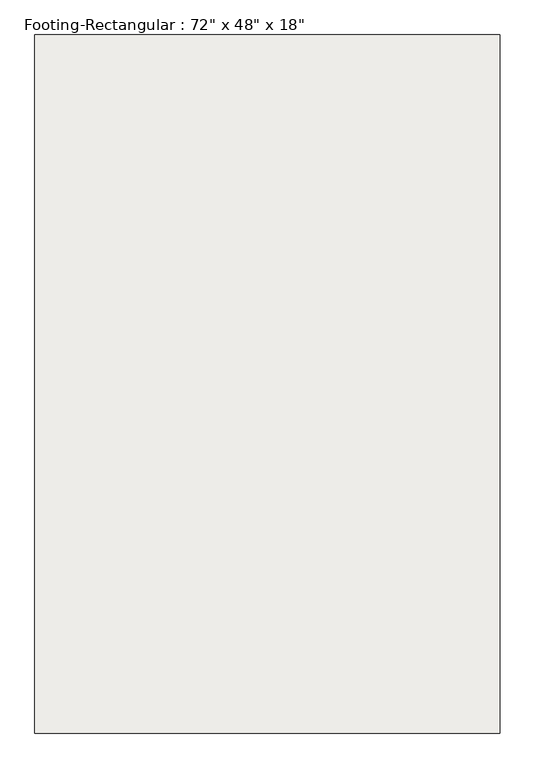
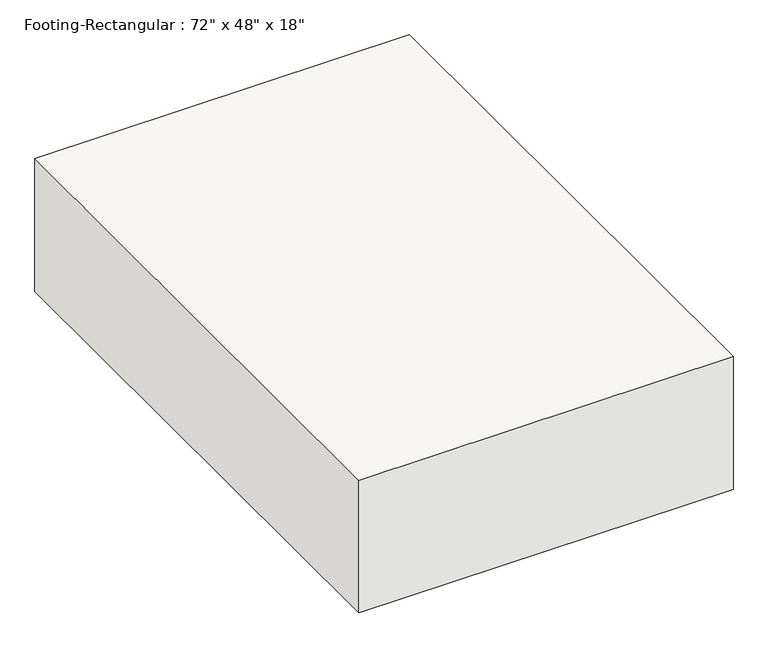
"""IFC4 building model written with IfcOpenShell, lengths in millimetres: slab geometry."""

from ifc_helpers import new_model, si_unit, frame, origin, place, context, project, spatial, polyline, outline, extrude, source, transform, mapped, element, save


def slab_5ba74754(model_context):
    return source(origin(), model_context, "Body", "SweptSolid", [
        extrude(outline(polyline([(609.6, 914.4), (609.6, -914.4), (-609.6, -914.4), (-609.6, 914.4), (609.6, 914.4)])), frame((0.0, 0.0, -457.2), z_axis=(0.0, 0.0, 1.0), x_axis=(1.0, 0.0, 0.0)), (0.0, 0.0, 1.0), 457.2),
    ])


if __name__ == "__main__":
    model = new_model("IFC4")
    model_context = context("Model", 3, world=origin())
    ifc_project = project(units=[si_unit("LENGTHUNIT", "METRE", prefix="MILLI")], contexts=[model_context])
    site = spatial("IfcSite", under=ifc_project)
    building = spatial("IfcBuilding", under=site)
    placement = place(None, origin())
    slab_shape = slab_5ba74754(model_context)
    element("IfcSlab", 1, ObjectType="Footing-Rectangular : 72\" x 48\" x 18\"", at=placement, inside=building, context=model_context, shape_type="MappedRepresentation", body=[
        mapped(slab_shape, transform((0.0, 0.0, 0.0), x_axis=(1.0, 0.0, 0.0), y_axis=(0.0, 1.0, 0.0), z_axis=(0.0, 0.0, 1.0))),
    ])
    save(model, "model.ifc")

# Revit data of these elements
# Type "Footing-Rectangular : 72\" x 48\" x 18\""
#   Assembly Code = "A1010100"
#   Width = 4' - 0"
#   Length = 6' - 0"
#   Foundation Thickness = 1' - 6"
#   Structural Material [instance default] = Concrete, Cast-in-Place gray
# Element 1 (IfcSlab, "Footing-Rectangular : 72\" x 48\" x 18\"")
#   Materials on its faces: "Concrete, Cast-in-Place gray"
# Materials
#   "Concrete, Cast-in-Place gray": class "Concrete", colour RGB 192 192 192, transparency 0, Description = "Cast-in-place concrete", Cost = 0
